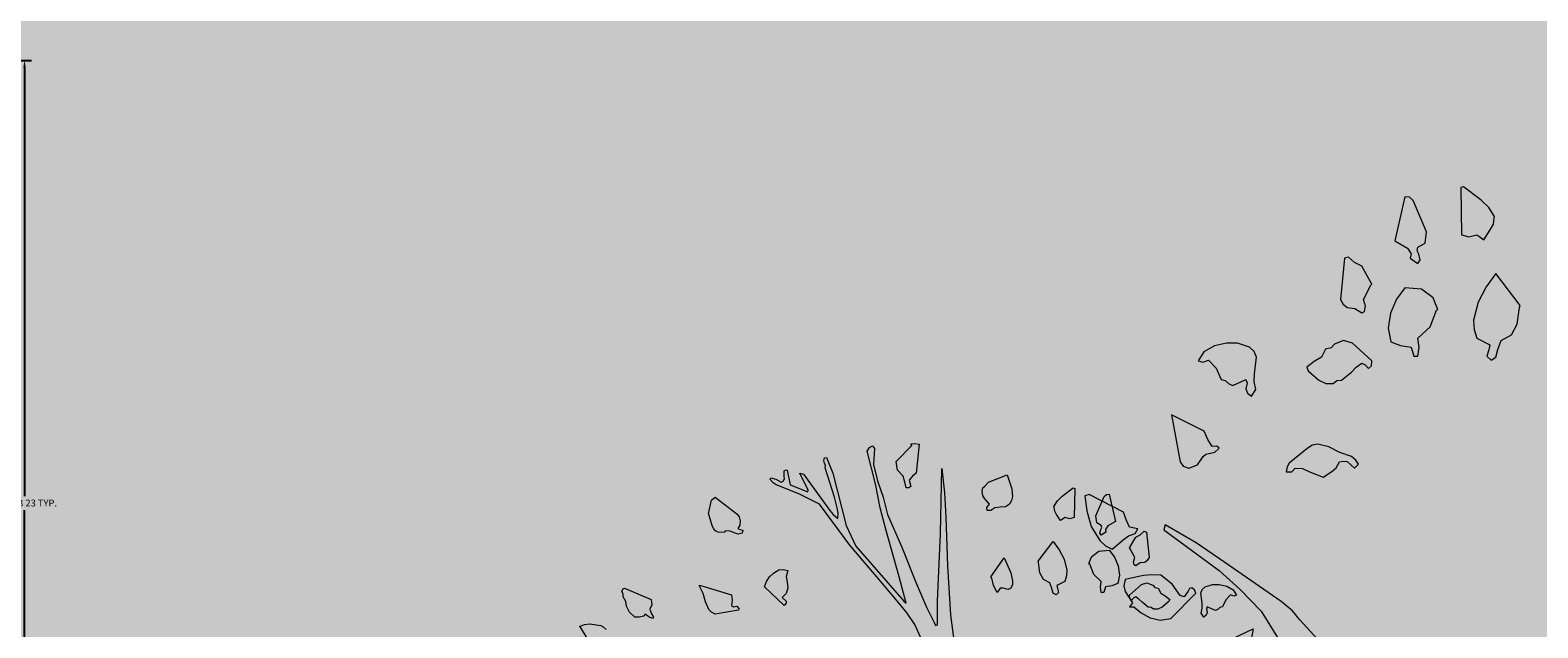
# Model space of a CAD drawing. Units: inches. Extents: x 84 to 1044, y -280 to 906.
# Tile 25 of 105: x 700 to 739, y -101 to -86. Entities that reach past the tile are written whole.
import ezdxf

# ---------------------------------------------------------------- set-up
doc = ezdxf.new("R2010")
doc.units = ezdxf.units.IN
doc.layers.add('A-ANNO-DIMS', color=2, linetype='Continuous', lineweight=18)
doc.layers.add('L-PLNT', color=114, linetype='Continuous', lineweight=15)
doc.layers.add('L-PLNT-PATT', color=9, linetype='Continuous', lineweight=9, true_color=0xafd9aa)
doc.styles.get("Standard").update_dxf_attribs({"font": 'arial.ttf'})
doc.dimstyles.get("Standard").update_dxf_attribs({"dimtxt": 0.18, "dimasz": 0.18, "dimexe": 0.18, "dimexo": 0.0625, "dimgap": 0.09, "dimtad": 0, "dimtih": 1, "dimtoh": 1, "dimdec": 4, "dimzin": 0, "dimdsep": 46, "dimtxsty": 'Standard', "dimcen": 0.09, "dimadec": 0, "dimazin": 0, "dimtfac": 1, "dimtdec": 4, "dimtofl": 0, "dimtmove": 0, "dimatfit": 3, "dimfxl": 1, "dimtolj": 1, "dimtzin": 0, "dimarcsym": 0})

# ---------------------------------------------------------------- blocks, each defined once
blk = doc.blocks.new('A$C37E508DF')
for p, q in [((0.7083, 1.5239), (0.7152, 1.5244)), ((0.7096, 1.5209), (0.7083, 1.5239)), ((0.7152, 1.5244), (0.7225, 1.5231)), ((0.7225, 1.5231), (0.7174, 1.4729)), ((0.6329, 1.5111), (0.6367, 1.5175)), ((0.6475, 1.4545), (0.6329, 1.5111)), ((0.6367, 1.5175), (0.6423, 1.5201)), ((0.6423, 1.5201), (0.6453, 1.5158)), ((0.6453, 1.5158), (0.644, 1.4879)), ((0.6826, 1.493), (0.7096, 1.5209)), ((0.5583, 1.4948), (0.5596, 1.4995)), ((0.5596, 1.4905), (0.5583, 1.4948)), ((0.5596, 1.4995), (0.563, 1.5003)), ((0.5613, 1.4862), (0.5596, 1.4905)), ((0.563, 1.5003), (0.5737, 1.4733)), ((0.6852, 1.4785), (0.6826, 1.493)), ((0.4897, 1.4772), (0.4935, 1.4789)), ((0.4897, 1.4678), (0.4897, 1.4772)), ((0.4935, 1.4789), (0.4952, 1.478)), ((0.4952, 1.478), (0.5004, 1.4532)), ((0.5608, 1.4823), (0.5613, 1.4862)), ((0.5767, 1.4317), (0.5608, 1.4823)), ((0.5737, 1.4733), (0.5814, 1.4437)), ((0.644, 1.4879), (0.6505, 1.46)), ((0.6946, 1.4682), (0.6852, 1.4785)), ((0.7589, 1.3691), (0.7615, 1.481)), ((0.7615, 1.481), (0.7658, 1.4395)), ((0.4657, 1.4622), (0.4669, 1.4652)), ((0.4708, 1.4566), (0.4657, 1.4622)), ((0.4669, 1.4652), (0.4755, 1.463)), ((0.4755, 1.463), (0.4845, 1.4575)), ((0.4845, 1.4575), (0.4884, 1.4596)), ((0.4884, 1.4596), (0.4905, 1.4635)), ((0.4905, 1.4635), (0.4897, 1.4678)), ((0.5313, 1.4437), (0.5167, 1.4729)), ((0.5167, 1.4729), (0.5231, 1.4716)), ((0.5231, 1.4716), (0.5686, 1.409)), ((0.6505, 1.46), (0.6603, 1.4317)), ((0.6976, 1.4579), (0.6946, 1.4682)), ((0.7002, 1.4476), (0.6976, 1.4579)), ((0.7109, 1.4682), (0.7053, 1.4609)), ((0.7053, 1.4609), (0.7083, 1.4502)), ((0.7174, 1.4729), (0.7109, 1.4682)), ((0.8357, 1.451), (0.8421, 1.4575)), ((0.8421, 1.4575), (0.8739, 1.4703)), ((0.8739, 1.4703), (0.882, 1.4463)), ((0.4764, 1.4532), (0.4708, 1.4566)), ((0.5154, 1.4373), (0.4764, 1.4532)), ((0.5004, 1.4532), (0.5308, 1.4412)), ((0.5308, 1.4412), (0.5313, 1.4437)), ((0.5814, 1.4437), (0.5969, 1.3833)), ((0.6552, 1.4137), (0.6475, 1.4545)), ((0.7049, 1.448), (0.7002, 1.4476)), ((0.7083, 1.4502), (0.7049, 1.448)), ((0.831, 1.4424), (0.8323, 1.4476)), ((0.8318, 1.4343), (0.831, 1.4424)), ((0.8323, 1.4476), (0.8357, 1.451)), ((0.882, 1.4463), (0.8829, 1.433)), ((0.9686, 1.4334), (0.9875, 1.4476)), ((0.9875, 1.4476), (0.9905, 1.4467)), ((0.9905, 1.4467), (0.9896, 1.3966)), ((0.3628, 1.4189), (0.3649, 1.4266)), ((0.3649, 1.4266), (0.3709, 1.4317)), ((0.3709, 1.4317), (0.4086, 1.403)), ((0.551, 1.4197), (0.5154, 1.4373)), ((0.5814, 1.4133), (0.5767, 1.4317)), ((0.6603, 1.4317), (0.668, 1.4021)), ((0.7658, 1.4395), (0.7684, 1.3979)), ((0.8353, 1.4292), (0.8318, 1.4343)), ((0.8434, 1.4197), (0.8353, 1.4292)), ((0.8816, 1.4262), (0.8781, 1.4197)), ((0.8829, 1.433), (0.8816, 1.4262)), ((0.9545, 1.4159), (0.9605, 1.4257)), ((0.9605, 1.4257), (0.9686, 1.4334)), ((1.0269, 1.3996), (1.0411, 1.433)), ((1.0411, 1.433), (1.045, 1.4365)), ((1.045, 1.4365), (1.0497, 1.4369)), ((1.0497, 1.4369), (1.0604, 1.3901)), ((0.3598, 1.403), (0.3628, 1.4189)), ((0.6029, 1.3494), (0.551, 1.4197)), ((0.5827, 1.4043), (0.5814, 1.4133)), ((0.6655, 1.3743), (0.6552, 1.4137)), ((0.8391, 1.4141), (0.8434, 1.4197)), ((0.8395, 1.4086), (0.8391, 1.4141)), ((0.8528, 1.4137), (0.846, 1.4086)), ((0.8619, 1.4146), (0.8528, 1.4137)), ((0.8709, 1.4154), (0.8619, 1.4146)), ((0.8781, 1.4197), (0.8709, 1.4154)), ((0.9549, 1.4146), (0.9545, 1.4159)), ((0.9558, 1.4077), (0.9549, 1.4146)), ((0.3602, 1.4021), (0.3598, 1.403)), ((0.364, 1.3888), (0.3602, 1.4021)), ((0.4086, 1.403), (0.4125, 1.3979)), ((0.4125, 1.3979), (0.4142, 1.391)), ((0.5686, 1.409), (0.5741, 1.4021)), ((0.5741, 1.4021), (0.5823, 1.3953)), ((0.5823, 1.3953), (0.5827, 1.4043)), ((0.668, 1.4021), (0.6925, 1.3455)), ((0.7684, 1.3979), (0.771, 1.3134)), ((0.846, 1.4086), (0.8395, 1.4086)), ((0.9592, 1.4017), (0.9558, 1.4077)), ((0.966, 1.3914), (0.9592, 1.4017)), ((0.9703, 1.3944), (0.966, 1.3914)), ((0.9733, 1.3966), (0.9703, 1.3944)), ((0.9819, 1.3944), (0.9733, 1.3966)), ((0.9896, 1.3966), (0.9819, 1.3944)), ((1.0282, 1.3876), (1.0269, 1.3996)), ((0.3657, 1.3828), (0.364, 1.3888)), ((0.3683, 1.3781), (0.3657, 1.3828)), ((0.3718, 1.3738), (0.3683, 1.3781)), ((0.4134, 1.3837), (0.4099, 1.3781)), ((0.4099, 1.3781), (0.4134, 1.376)), ((0.4142, 1.391), (0.4134, 1.3837)), ((0.5969, 1.3833), (0.6132, 1.3472)), ((1.0359, 1.3833), (1.0282, 1.3876)), ((1.0351, 1.376), (1.0368, 1.3794)), ((1.0368, 1.3794), (1.0359, 1.3833)), ((1.0471, 1.3824), (1.0432, 1.3764)), ((1.0604, 1.3901), (1.0471, 1.3824)), ((0.3765, 1.3713), (0.3718, 1.3738)), ((0.3872, 1.3708), (0.3765, 1.3713)), ((0.3885, 1.3738), (0.3872, 1.3708)), ((0.3971, 1.3734), (0.3885, 1.3738)), ((0.4039, 1.3704), (0.3971, 1.3734)), ((0.4108, 1.3683), (0.4039, 1.3704)), ((0.4176, 1.37), (0.4108, 1.3683)), ((0.4134, 1.376), (0.4189, 1.3751)), ((0.4189, 1.3751), (0.4176, 1.37)), ((0.6882, 1.2949), (0.6655, 1.3743)), ((0.7538, 1.2529), (0.7589, 1.3691)), ((1.0334, 1.37), (1.0351, 1.376)), ((1.0359, 1.3661), (1.0334, 1.37)), ((1.0441, 1.3717), (1.0359, 1.3661)), ((1.0432, 1.3764), (1.0441, 1.3717)), ((1.0848, 1.3443), (1.0955, 1.3631)), ((1.0955, 1.3631), (1.1033, 1.367)), ((1.1033, 1.367), (1.1097, 1.373)), ((1.1097, 1.373), (1.114, 1.3717)), ((1.114, 1.3717), (1.1183, 1.328)), ((0.6595, 1.2829), (0.6029, 1.3494)), ((0.6132, 1.3472), (0.6959, 1.2529)), ((0.6925, 1.3455), (0.7161, 1.2868)), ((0.9274, 1.3215), (0.9532, 1.3554)), ((0.9532, 1.3554), (0.9635, 1.3413)), ((0.9635, 1.3413), (0.9721, 1.325)), ((1.0171, 1.3232), (1.0197, 1.3297)), ((1.0197, 1.3297), (1.0321, 1.3387)), ((1.0321, 1.3387), (1.0497, 1.3404)), ((1.0497, 1.3404), (1.0587, 1.3284)), ((1.0861, 1.343), (1.0848, 1.3443)), ((1.0938, 1.328), (1.0861, 1.343)), ((0.771, 1.3134), (0.7761, 1.2285)), ((0.846, 1.2949), (0.8687, 1.3271)), ((0.8687, 1.3271), (0.8803, 1.3014)), ((0.9279, 1.3194), (0.9274, 1.3215)), ((0.9305, 1.3018), (0.9279, 1.3194)), ((0.9721, 1.325), (0.9768, 1.3061)), ((1.0149, 1.3172), (1.0171, 1.3232)), ((1.0162, 1.3164), (1.0149, 1.3172)), ((1.0231, 1.2988), (1.0162, 1.3164)), ((1.0587, 1.3284), (1.0651, 1.3134)), ((1.0651, 1.3134), (1.0677, 1.2975)), ((1.0917, 1.3207), (1.0938, 1.328)), ((1.0925, 1.3151), (1.0917, 1.3207)), ((1.0955, 1.3138), (1.0925, 1.3151)), ((1.1028, 1.3185), (1.0955, 1.3138)), ((1.111, 1.3194), (1.1028, 1.3185)), ((1.1153, 1.3228), (1.111, 1.3194)), ((1.1183, 1.328), (1.1153, 1.3228)), ((0.4648, 1.2945), (0.4717, 1.3009)), ((0.4717, 1.3009), (0.4807, 1.3065)), ((0.4807, 1.3065), (0.4884, 1.3074)), ((0.4884, 1.3074), (0.4965, 1.3057)), ((0.4965, 1.3057), (0.4935, 1.2954)), ((0.8803, 1.3014), (0.8833, 1.2872)), ((0.9365, 1.2902), (0.9305, 1.3018)), ((0.9768, 1.3061), (0.9763, 1.2962)), ((1.0359, 1.2868), (1.0231, 1.2988)), ((1.0677, 1.2975), (1.0647, 1.2829)), ((0.4562, 1.2774), (0.4597, 1.2868)), ((0.4597, 1.2868), (0.4648, 1.2945)), ((0.4935, 1.2954), (0.4948, 1.2855)), ((0.4948, 1.2855), (0.4961, 1.2756)), ((0.6865, 1.2508), (0.6595, 1.2829)), ((0.7002, 1.2495), (0.6882, 1.2949)), ((0.7161, 1.2868), (0.7349, 1.2422)), ((0.8473, 1.2924), (0.846, 1.2949)), ((0.8507, 1.2795), (0.8473, 1.2924)), ((0.8833, 1.2872), (0.8829, 1.2808)), ((0.9476, 1.2842), (0.9365, 1.2902)), ((0.951, 1.2748), (0.9476, 1.2842)), ((0.9733, 1.2868), (0.9596, 1.2799)), ((0.9763, 1.2962), (0.9733, 1.2868)), ((1.0347, 1.2769), (1.0359, 1.2868)), ((1.0647, 1.2829), (1.0544, 1.2791)), ((1.0848, 1.2628), (1.1054, 1.2817)), ((1.1054, 1.2817), (1.1148, 1.2842)), ((1.1148, 1.2842), (1.1247, 1.2804)), ((1.2147, 1.2774), (1.2276, 1.2817)), ((1.2276, 1.2817), (1.2392, 1.2817)), ((1.2392, 1.2817), (1.2521, 1.2787)), ((0.2101, 1.2696), (0.2127, 1.2744)), ((0.2127, 1.2654), (0.2101, 1.2696)), ((0.2127, 1.2744), (0.2152, 1.2752)), ((0.2127, 1.2602), (0.2127, 1.2654)), ((0.2152, 1.2752), (0.2611, 1.2559)), ((0.3439, 1.2804), (0.3992, 1.2636)), ((0.3439, 1.2787), (0.3439, 1.2804)), ((0.3507, 1.2662), (0.3439, 1.2787)), ((0.3546, 1.2516), (0.3507, 1.2662)), ((0.4897, 1.2452), (0.4562, 1.2774)), ((0.4935, 1.2658), (0.4867, 1.2589)), ((0.4961, 1.2756), (0.4935, 1.2658)), ((0.8567, 1.2679), (0.8507, 1.2795)), ((0.8619, 1.2752), (0.8567, 1.2679)), ((0.867, 1.2752), (0.8619, 1.2752)), ((0.8713, 1.2739), (0.867, 1.2752)), ((0.8756, 1.2726), (0.8713, 1.2739)), ((0.8799, 1.2744), (0.8756, 1.2726)), ((0.8829, 1.2808), (0.8799, 1.2744)), ((0.9532, 1.2666), (0.951, 1.2748)), ((0.9583, 1.2636), (0.9532, 1.2666)), ((0.9626, 1.2679), (0.9583, 1.2636)), ((0.9596, 1.2799), (0.9605, 1.2744)), ((0.9605, 1.2744), (0.9626, 1.2679)), ((1.0359, 1.2679), (1.0347, 1.2769)), ((1.0402, 1.2679), (1.0359, 1.2679)), ((1.0432, 1.2774), (1.0402, 1.2679)), ((1.0544, 1.2791), (1.0432, 1.2774)), ((1.1247, 1.2804), (1.1281, 1.2765)), ((1.1281, 1.2765), (1.1341, 1.2752)), ((1.1341, 1.2752), (1.1384, 1.2666)), ((1.1384, 1.2666), (1.1461, 1.2619)), ((1.2075, 1.2666), (1.21, 1.2726)), ((1.2096, 1.2491), (1.2075, 1.2666)), ((1.21, 1.2726), (1.2147, 1.2774)), ((1.2521, 1.2787), (1.2632, 1.2722)), ((1.2632, 1.2722), (1.2692, 1.2628)), ((0.2174, 1.2521), (0.2127, 1.2602)), ((0.2182, 1.2443), (0.2174, 1.2521)), ((0.2611, 1.2559), (0.262, 1.2465)), ((0.3602, 1.2383), (0.3546, 1.2516)), ((0.3992, 1.2636), (0.4005, 1.2546)), ((0.4005, 1.2546), (0.3992, 1.2452)), ((0.4867, 1.2589), (0.4935, 1.2529)), ((0.4931, 1.2491), (0.4897, 1.2452)), ((0.4935, 1.2529), (0.4931, 1.2491)), ((0.7015, 1.2323), (0.6865, 1.2508)), ((0.6959, 1.2529), (0.7002, 1.2495)), ((0.7538, 1.2122), (0.7538, 1.2529)), ((1.0852, 1.2576), (1.0848, 1.2628)), ((1.0883, 1.2546), (1.0852, 1.2576)), ((1.0921, 1.2585), (1.0883, 1.2546)), ((1.0955, 1.2602), (1.0921, 1.2585)), ((1.1015, 1.2559), (1.0955, 1.2602)), ((1.1063, 1.2508), (1.1015, 1.2559)), ((1.117, 1.2422), (1.1063, 1.2508)), ((1.1526, 1.2521), (1.141, 1.2422)), ((1.1461, 1.2619), (1.1539, 1.2559)), ((1.1539, 1.2559), (1.1526, 1.2521)), ((1.21, 1.2409), (1.2096, 1.2491)), ((1.2503, 1.2551), (1.2448, 1.2431)), ((1.2585, 1.2636), (1.2503, 1.2551)), ((1.2645, 1.2615), (1.2585, 1.2636)), ((1.2692, 1.2628), (1.2645, 1.2615)), ((0.2234, 1.2336), (0.2182, 1.2443)), ((0.2328, 1.2251), (0.2234, 1.2336)), ((0.262, 1.2465), (0.2586, 1.2388)), ((0.2586, 1.2388), (0.2611, 1.2319)), ((0.3649, 1.2336), (0.3602, 1.2383)), ((0.3709, 1.2306), (0.3649, 1.2336)), ((0.4112, 1.2375), (0.3709, 1.2306)), ((0.3992, 1.2452), (0.4026, 1.2431)), ((0.4026, 1.2431), (0.4086, 1.2443)), ((0.4086, 1.2443), (0.4121, 1.2401)), ((0.4121, 1.2401), (0.4112, 1.2375)), ((0.7349, 1.2422), (0.7482, 1.216)), ((1.1221, 1.2418), (1.117, 1.2422)), ((1.126, 1.2388), (1.1221, 1.2418)), ((1.1337, 1.2388), (1.126, 1.2388)), ((1.141, 1.2422), (1.1337, 1.2388)), ((1.2079, 1.2323), (1.21, 1.2409)), ((1.2186, 1.2332), (1.2169, 1.2285)), ((1.2186, 1.2431), (1.2173, 1.2392)), ((1.2173, 1.2392), (1.2186, 1.2332)), ((1.2285, 1.2383), (1.2186, 1.2431)), ((1.2328, 1.2366), (1.2285, 1.2383)), ((1.2371, 1.2388), (1.2328, 1.2366)), ((1.2405, 1.2418), (1.2371, 1.2388)), ((1.2448, 1.2431), (1.2405, 1.2418)), ((0.2401, 1.2251), (0.2328, 1.2251)), ((0.2474, 1.2268), (0.2401, 1.2251)), ((0.2504, 1.2306), (0.2474, 1.2268)), ((0.2568, 1.2255), (0.2504, 1.2306)), ((0.2633, 1.2229), (0.2568, 1.2255)), ((0.2611, 1.2319), (0.265, 1.2251)), ((0.265, 1.2251), (0.2633, 1.2229)), ((0.7148, 1.2126), (0.7015, 1.2323)), ((0.7761, 1.2285), (0.7821, 1.1856)), ((1.2126, 1.2251), (1.2079, 1.2323)), ((1.2169, 1.2285), (1.2126, 1.2251)), ((0.1376, 1.2092), (0.1458, 1.2126)), ((0.1389, 1.2079), (0.1376, 1.2092)), ((0.1505, 1.189), (0.1389, 1.2079)), ((0.1458, 1.2126), (0.1548, 1.2135)), ((0.1548, 1.2135), (0.1741, 1.2109)), ((0.1741, 1.2109), (0.1784, 1.2083)), ((0.1784, 1.2083), (0.1831, 1.204)), ((0.7246, 1.1908), (0.7148, 1.2126)), ((0.7482, 1.216), (0.7508, 1.2109)), ((0.7508, 1.2109), (0.7538, 1.2122)), ((1.2628, 1.1882), (1.2975, 1.2053)), ((1.2975, 1.2053), (1.2885, 1.1556)), ((1.2589, 1.1792), (1.2628, 1.1882)), ((1.1187, 1.1655), (1.1307, 1.1714)), ((1.1307, 1.1714), (1.1423, 1.1744)), ((1.1423, 1.1744), (1.1483, 1.1732)), ((1.1483, 1.1732), (1.1539, 1.1693)), ((1.1539, 1.1693), (1.1727, 1.1543)), ((1.2469, 1.1702), (1.2495, 1.1723)), ((1.2478, 1.1693), (1.2469, 1.1702)), ((1.2516, 1.1659), (1.2478, 1.1693)), ((1.2495, 1.1723), (1.2546, 1.1719)), ((1.2546, 1.1719), (1.2589, 1.1792)), ((1.099, 1.153), (1.102, 1.1573)), ((1.1033, 1.1487), (1.099, 1.153)), ((1.102, 1.1573), (1.1063, 1.1612)), ((1.111, 1.156), (1.1033, 1.1487)), ((1.1063, 1.1612), (1.1187, 1.1655)), ((1.1153, 1.1564), (1.111, 1.156)), ((1.1191, 1.1556), (1.1153, 1.1564)), ((1.1226, 1.1492), (1.1191, 1.1556)), ((1.1727, 1.1543), (1.1749, 1.1504)), ((1.2563, 1.1646), (1.2516, 1.1659)), ((1.2611, 1.1637), (1.2563, 1.1646)), ((1.2641, 1.1612), (1.2611, 1.1637)), ((1.2701, 1.1522), (1.2641, 1.1612)), ((1.2885, 1.1556), (1.2851, 1.1509)), ((1.1273, 1.1453), (1.1226, 1.1492)), ((1.1367, 1.1393), (1.1273, 1.1453)), ((1.1517, 1.1453), (1.1367, 1.1393)), ((1.1586, 1.1483), (1.1517, 1.1453)), ((1.1663, 1.1487), (1.1586, 1.1483)), ((1.1697, 1.1449), (1.1663, 1.1487)), ((1.1757, 1.1449), (1.1697, 1.1449)), ((1.1749, 1.1504), (1.1757, 1.1449)), ((1.2791, 1.1487), (1.2701, 1.1522)), ((1.2851, 1.1509), (1.2791, 1.1487)), ((1.3485, 1.102), (1.385, 1.1209)), ((1.385, 1.1209), (1.3897, 1.1196)), ((1.3897, 1.1196), (1.3875, 1.1037)), ((1.3421, 1.0861), (1.3455, 1.0934)), ((1.3455, 1.0934), (1.3485, 1.102)), ((1.3875, 1.1037), (1.3828, 1.087)), ((1.3057, 1.0835), (1.2469, 1.0402)), ((1.2713, 1.0694), (1.3044, 1.0887)), ((1.3044, 1.0887), (1.3057, 1.0835)), ((1.3335, 1.0844), (1.3421, 1.0861)), ((1.3361, 1.0793), (1.3335, 1.0844)), ((1.3434, 1.0771), (1.3361, 1.0793)), ((1.349, 1.0728), (1.3434, 1.0771)), ((1.3605, 1.063), (1.349, 1.0728)), ((1.3828, 1.087), (1.3738, 1.072)), ((1.2409, 1.0488), (1.2713, 1.0694)), ((1.3678, 1.0664), (1.3605, 1.063)), ((1.3738, 1.072), (1.3678, 1.0664)), ((1.1813, 1.0072), (1.2409, 1.0488)), ((1.2469, 1.0402), (1.2246, 1.0201)), ((1.2885, 1.0136), (1.2971, 1.0257)), ((1.2971, 1.0257), (1.3091, 1.0351)), ((1.3091, 1.0351), (1.3185, 1.0355)), ((1.3185, 1.0355), (1.3275, 1.0347)), ((1.3275, 1.0347), (1.3468, 1.0308)), ((1.3468, 1.0308), (1.3481, 1.0239)), ((1.2246, 1.0201), (1.2023, 0.9969)), ((1.2718, 1.0162), (1.2731, 1.0197)), ((1.2984, 0.9892), (1.2718, 1.0162)), ((1.2731, 1.0197), (1.2761, 1.0218)), ((1.2761, 1.0218), (1.2786, 1.0209)), ((1.2786, 1.0209), (1.2799, 1.0184)), ((1.2799, 1.0184), (1.2842, 1.0124)), ((1.2842, 1.0124), (1.2885, 1.0136)), ((1.3468, 1.018), (1.3391, 1.0059)), ((1.3481, 1.0239), (1.3468, 1.018)), ((1.1612, 0.9879), (1.1693, 0.9974)), ((1.1693, 0.9974), (1.1813, 1.0072)), ((1.2023, 0.9969), (1.1852, 0.9691)), ((1.3297, 0.9952), (1.3202, 0.9901)), ((1.3378, 1.0016), (1.3297, 0.9952)), ((1.3421, 1.0016), (1.3378, 1.0016)), ((1.3391, 1.0059), (1.3421, 1.0016)), ((1.1311, 0.9549), (1.1612, 0.9879)), ((1.3095, 0.9875), (1.2984, 0.9892)), ((1.3202, 0.9901), (1.3095, 0.9875))]:
    blk.add_line(p, q)
blk = doc.blocks.new('*D30')
at = {"layer": 'A-ANNO-DIMS', "color": 0, "lineweight": -2, "transparency": 16777216}
for p, q in [((696.303, -86.54), (699.895, -86.54)), ((699.715, -86.72), (699.715, -97.938)), ((699.715, -109.523), (699.715, -98.305)), ((696.303, -109.703), (699.895, -109.703))]:
    blk.add_line(p, q, dxfattribs=at)
at = {"layer": 'A-ANNO-DIMS', "color": 0, "transparency": 16777216}
for points in [[(699.685, -86.72), (699.745, -86.72), (699.715, -86.54)], [(699.685, -109.523), (699.745, -109.523), (699.715, -109.703)]]:
    blk.add_solid(points, dxfattribs=at)
at = {"layer": 'Defpoints', "color": 0, "transparency": 16777216}
for p in [(696.24, -86.54), (699.715, -86.54), (696.24, -109.703)]:
    blk.add_point(p, dxfattribs=at)
at = {"layer": 'A-ANNO-DIMS', "color": 0, "transparency": 16777216, "insert": (699.715, -98.121), "char_height": 0.18, "attachment_point": 5}
blk.add_mtext('\\A1;SHRUB 23 TYP.', dxfattribs=at)

msp = doc.modelspace()

# ---------------------------------------------------------------- hatches: boundary and pattern name
at = {"layer": 'L-PLNT-PATT', "transparency": 33554597}
h = msp.add_hatch(color=256, dxfattribs=at)
h.dxf.hatch_style = 1
h.paths.add_polyline_path([(791.074, 31.12), (791.074, 91.12), (743.074, 91.12), (674.074, 91.12), (674.074, 31.12), (650.074, 31.12), (650.074, -112.88), (983.074, -112.88), (983.074, -64.88), (791.074, -64.88)])

# ---------------------------------------------------------------- block references
at = {"layer": 'L-PLNT'}
for p, xscale, yscale, zscale in [((761.712, -125.52), -24.64361536662419, 24.64361536662419, 24.64361536662419), ((712.152, -119.725, 0), 15.19586232982809, 15.19586232982809, 15.19586232982809)]:
    msp.add_blockref('A$C37E508DF', p, dxfattribs=dict(at, xscale=xscale, yscale=yscale, zscale=zscale))

# ---------------------------------------------------------------- dimensions: what is measured, and where the dimension line sits
at = {"layer": 'A-ANNO-DIMS'}
dim = msp.add_linear_dim(base=(699.715, -86.54), p1=(696.24, -109.703), p2=(696.24, -86.54), angle=90, text='SHRUB <> TYP.', dimstyle='Standard', override={"dimdec": 0, "dimlfac": 1, "dimrnd": 0, "dimzin": 0, "dimdsep": 46, "dimlunit": 2}, dxfattribs=at)
dim.commit()
dim.dimension.update_dxf_attribs({"geometry": '*D30', "text_midpoint": (699.715, -98.121)})

doc.saveas('drawing.dxf')
